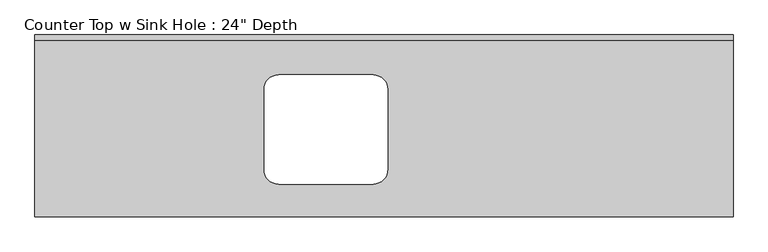
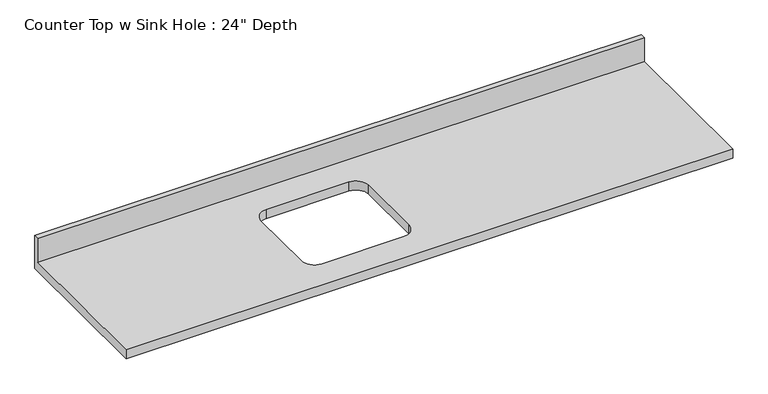
"""IFC4 building model written with IfcOpenShell, lengths in millimetres: furniture geometry."""

from ifc_helpers import new_model, si_unit, frame, origin, place, context, project, spatial, polyline, circle_curve, source, transform, mapped, element, save
from ifc_brep_helpers import plane_surface, revolved_surface, advanced_brep


def furniture_8d292e24(model_context):
    return source(origin(), model_context, "Body", "AdvancedBrep", [
        advanced_brep(
        [(-1200.4622951, -635.0, 914.4), (1237.9377049, -635.0, 914.4), (1237.9377049, -19.05, 914.4), (-1200.4622951, -19.05, 914.4), (-349.5622951, -139.7, 914.4), (-19.3622951, -139.7, 914.4), (31.4377049, -190.5, 914.4), (31.4377049, -469.9, 914.4), (-19.3622951, -520.7, 914.4), (-349.5622951, -520.7, 914.4), (-400.3622951, -469.9, 914.4), (-400.3622951, -190.5, 914.4), (1237.9377049, 0.0, 876.3), (1237.9377049, -635.0, 876.3), (-1200.4622951, -635.0, 876.3), (-1200.4622951, 0.0, 876.3), (-19.3622951, -139.7, 876.3), (-349.5622951, -139.7, 876.3), (-400.3622951, -190.5, 876.3), (-400.3622951, -469.9, 876.3), (-349.5622951, -520.7, 876.3), (-19.3622951, -520.7, 876.3), (31.4377049, -469.9, 876.3), (31.4377049, -190.5, 876.3), (-1200.4622951, 0.0, 1016.0), (1237.9377049, 0.0, 1016.0), (-1200.4622951, -19.05, 1016.0), (1237.9377049, -19.05, 1016.0)],
        [
            (0, 1),
            (1, 2),
            (2, 3),
            (3, 0),
            (4, 5),
            (5, 6, circle_curve(frame((-19.3622951, -190.5, 914.4), z_axis=(0.0, 0.0, -1.0), x_axis=(1.0, 0.0, 0.0)), 50.8)),
            (6, 7),
            (7, 8, circle_curve(frame((-19.3622951, -469.9, 914.4), z_axis=(0.0, 0.0, -1.0), x_axis=(1.0, 0.0, 0.0)), 50.8)),
            (8, 9),
            (9, 10, circle_curve(frame((-349.5622951, -469.9, 914.4), z_axis=(0.0, 0.0, -1.0), x_axis=(1.0, 0.0, 0.0)), 50.8)),
            (10, 11),
            (11, 4, circle_curve(frame((-349.5622951, -190.5, 914.4), z_axis=(0.0, 0.0, -1.0), x_axis=(1.0, 0.0, 0.0)), 50.8)),
            (12, 13),
            (13, 14),
            (14, 15),
            (15, 12),
            (16, 17),
            (17, 18, circle_curve(frame((-349.5622951, -190.5, 876.3), z_axis=(0.0, 0.0, 1.0), x_axis=(1.0, 0.0, 0.0)), 50.8)),
            (18, 19),
            (19, 20, circle_curve(frame((-349.5622951, -469.9, 876.3), z_axis=(0.0, 0.0, 1.0), x_axis=(1.0, 0.0, 0.0)), 50.8)),
            (20, 21),
            (21, 22, circle_curve(frame((-19.3622951, -469.9, 876.3), z_axis=(0.0, 0.0, 1.0), x_axis=(1.0, 0.0, 0.0)), 50.8)),
            (22, 23),
            (23, 16, circle_curve(frame((-19.3622951, -190.5, 876.3), z_axis=(0.0, 0.0, 1.0), x_axis=(1.0, 0.0, 0.0)), 50.8)),
            (15, 24),
            (24, 25),
            (25, 12),
            (14, 0),
            (3, 26),
            (26, 24),
            (13, 1),
            (25, 27),
            (27, 2),
            (4, 17),
            (16, 5),
            (11, 18),
            (10, 19),
            (9, 20),
            (8, 21),
            (7, 22),
            (6, 23),
            (26, 27),
        ],
        [
            plane_surface(frame((-1200.4622951, 0.0, 914.4), z_axis=(0.0, 0.0, 1.0), x_axis=(-1.0, 0.0, 0.0))),
            plane_surface(frame((-1200.4622951, 0.0, 876.3), z_axis=(0.0, 0.0, -1.0), x_axis=(1.0, 0.0, 0.0))),
            plane_surface(frame((1237.9377049, 0.0, 914.4), z_axis=(0.0, 1.0, 0.0), x_axis=(0.0, 0.0, -1.0))),
            plane_surface(frame((-1200.4622951, 0.0, 914.4), z_axis=(-1.0, 0.0, 0.0), x_axis=(0.0, 0.0, -1.0))),
            plane_surface(frame((-1200.4622951, -635.0, 914.4), z_axis=(0.0, -1.0, 0.0), x_axis=(0.0, 0.0, -1.0))),
            plane_surface(frame((1237.9377049, -635.0, 914.4), z_axis=(1.0, 0.0, 0.0), x_axis=(0.0, 0.0, -1.0))),
            plane_surface(frame((-19.3622951, -139.7, 914.4), z_axis=(0.0, -1.0, 0.0), x_axis=(0.0, 0.0, -1.0))),
            revolved_surface(polyline([(-298.76229509999996, -190.5, 914.4), (-298.76229509999996, -190.5, 876.3)]), (-349.5622951, -190.5, 876.3), (0.0, 0.0, 1.0)),
            plane_surface(frame((-400.3622951, -190.5, 914.4), z_axis=(1.0, 0.0, 0.0), x_axis=(0.0, 0.0, -1.0))),
            revolved_surface(polyline([(-298.76229509999996, -469.9, 914.4), (-298.76229509999996, -469.9, 876.3)]), (-349.5622951, -469.9, 876.3), (0.0, 0.0, 1.0)),
            plane_surface(frame((-349.5622951, -520.7, 914.4), z_axis=(0.0, 1.0, 0.0), x_axis=(0.0, 0.0, -1.0))),
            revolved_surface(polyline([(31.437704899999996, -469.9, 914.4), (31.437704899999996, -469.9, 876.3)]), (-19.3622951, -469.9, 876.3), (0.0, 0.0, 1.0)),
            plane_surface(frame((31.4377049, -469.9, 914.4), z_axis=(-1.0, 0.0, 0.0), x_axis=(0.0, 0.0, -1.0))),
            revolved_surface(polyline([(31.437704899999996, -190.5, 914.4), (31.437704899999996, -190.5, 876.3)]), (-19.3622951, -190.5, 876.3), (0.0, 0.0, 1.0)),
            plane_surface(frame((-1200.4622951, 0.0, 1016.0), z_axis=(0.0, 0.0, 1.0), x_axis=(0.0, -1.0, 0.0))),
            plane_surface(frame((-1200.4622951, -19.05, 1016.0), z_axis=(0.0, -1.0, 0.0), x_axis=(0.0, 0.0, -1.0))),
        ],
        [
            (0, [[1, 2, 3, 4], [5, 6, 7, 8, 9, 10, 11, 12]]),
            (1, [[13, 14, 15, 16], [17, 18, 19, 20, 21, 22, 23, 24]]),
            (2, [[-16, 25, 26, 27]]),
            (3, [[-15, 28, -4, 29, 30, -25]]),
            (4, [[-1, -28, -14, 31]]),
            (5, [[-13, -27, 32, 33, -2, -31]]),
            (6, [[34, -17, 35, -5]]),
            (7, [[-34, -12, 36, -18]]),
            (8, [[-36, -11, 37, -19]]),
            (9, [[-37, -10, 38, -20]]),
            (10, [[-38, -9, 39, -21]]),
            (11, [[-39, -8, 40, -22]]),
            (12, [[-40, -7, 41, -23]]),
            (13, [[-35, -24, -41, -6]]),
            (14, [[-30, 42, -32, -26]]),
            (15, [[-42, -29, -3, -33]]),
        ],
    ),
    ])


if __name__ == "__main__":
    model = new_model("IFC4")
    model_context = context("Model", 3, world=origin())
    ifc_project = project(units=[si_unit("LENGTHUNIT", "METRE", prefix="MILLI")], contexts=[model_context])
    site = spatial("IfcSite", under=ifc_project)
    building = spatial("IfcBuilding", under=site)
    placement = place(None, origin())
    furniture_shape = furniture_8d292e24(model_context)
    element("IfcFurniture", 1, ObjectType="Counter Top w Sink Hole : 24\" Depth", at=placement, inside=building, context=model_context, shape_type="MappedRepresentation", body=[
        mapped(furniture_shape, transform((0.0, 0.0, 0.0), x_axis=(1.0, 0.0, 0.0), y_axis=(0.0, 1.0, 0.0), z_axis=(0.0, 0.0, 1.0))),
    ])
    save(model, "model.ifc")

# Revit data of these elements
# Type "Counter Top w Sink Hole : 24\" Depth"
#   Assembly Code = "C1030400"
#   Counter Thickness = 0' - 1 1/2"
#   Depth = 2' - 1"
#   Height = 3' - 0"
#   Length [instance default] = 8' - 0"
#   Sink Location [instance default] = 2' - 0"
#   Sink Location To Wall [instance default] = 0' - 6"
#   Sink Opening Depth [instance default] = 1' - 3"
#   Sink Opening Width [instance default] = 2' - 3"
#   Counter Top Material = none
#   Default Elevation = 0
# Element 1 (IfcFurniture, "Counter Top w Sink Hole : 24\" Depth")
#   Sink Location = 3' - 4"
#   Sink Opening Depth = 1' - 2"
#   Sink Opening Width = 1' - 4"
#   Materials on its faces: "Counter Top"
# Materials
#   "Counter Top": class "Wood", colour RGB 226 177 128, transparency 0
